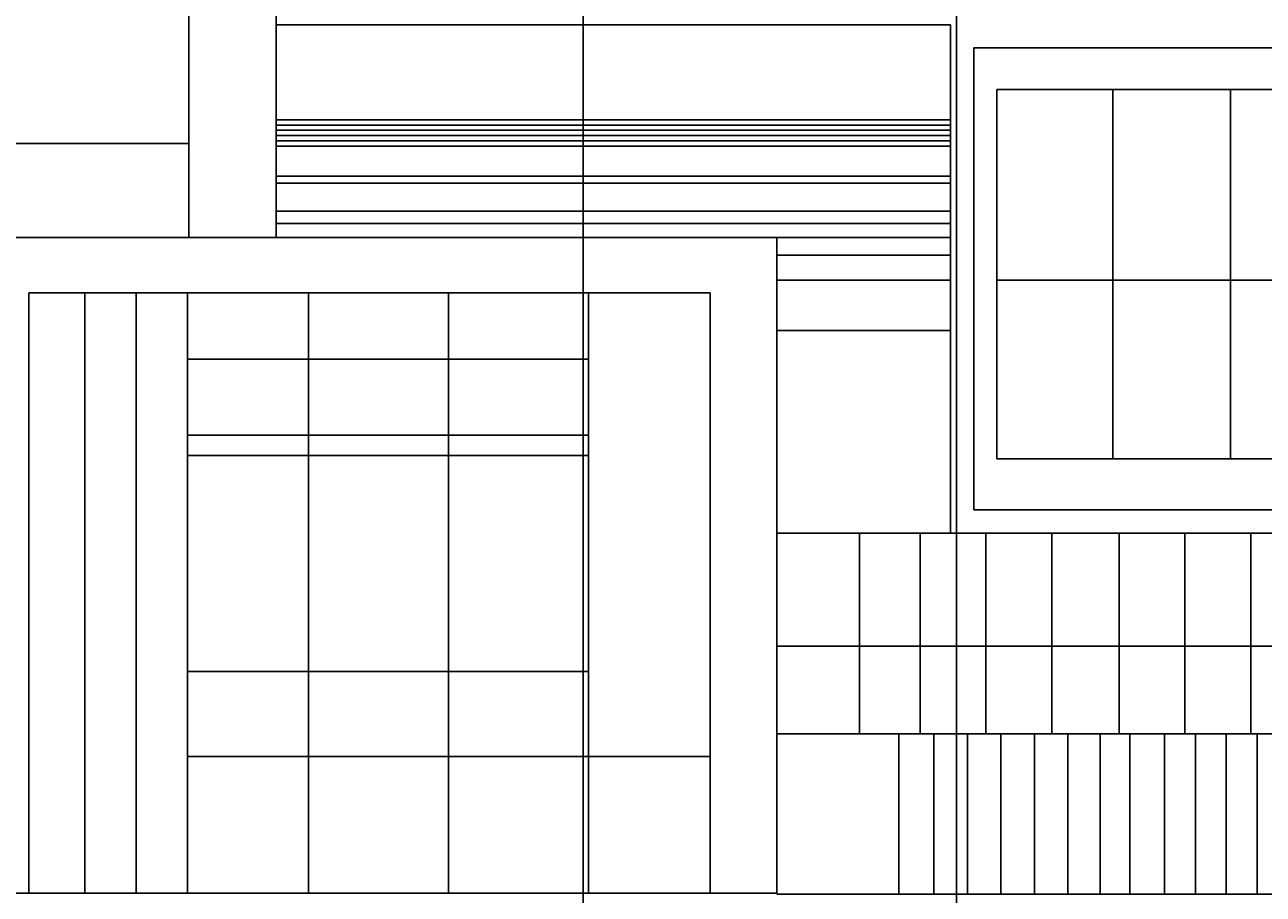
# Model space of a CAD drawing. Units: inches. Extents: x -117 to 121, y -77 to 40.
# Tile 29 of 45: x 9 to 34, y -8 to 10. Entities that reach past the tile are written whole.
import ezdxf

# ---------------------------------------------------------------- set-up
doc = ezdxf.new("R2010")
doc.units = ezdxf.units.IN
doc.header["$MEASUREMENT"] = 0
doc.layers.add('A-ANNO-DIMS', color=2, linetype='Continuous', lineweight=18)
doc.layers.add('A-ELEV', color=7, linetype='Continuous', lineweight=25)
doc.styles.get("Standard").update_dxf_attribs({"font": 'arial.ttf'})
doc.dimstyles.get("Standard").update_dxf_attribs({"dimtxt": 0.18, "dimasz": 0.18, "dimexe": 0.18, "dimexo": 0.0625, "dimgap": 0.09, "dimtad": 0, "dimtih": 1, "dimtoh": 1, "dimdec": 4, "dimzin": 0, "dimdsep": 46, "dimtxsty": 'Standard', "dimcen": 0.09, "dimadec": 0, "dimazin": 0, "dimtfac": 1, "dimtdec": 4, "dimtofl": 0, "dimtmove": 0, "dimatfit": 3, "dimfxl": 1, "dimtolj": 1, "dimtzin": 0, "dimarcsym": 0})

# ---------------------------------------------------------------- blocks, each defined once
blk = doc.blocks.new('*D32')
at = {"layer": 'A-ANNO-DIMS', "color": 0, "lineweight": -2, "transparency": 16777216}
for p, q in [((-3.85, -45.55), (-3.85, 38.61)), ((20.293, -45.55), (20.293, 38.61)), ((-3.67, 38.43), (7.757, 38.43)), ((20.113, 38.43), (8.686, 38.43))]:
    blk.add_line(p, q, dxfattribs=at)
at = {"layer": 'A-ANNO-DIMS', "color": 0, "transparency": 16777216}
for points in [[(-3.67, 38.46), (-3.67, 38.4), (-3.85, 38.43)], [(20.113, 38.46), (20.113, 38.4), (20.293, 38.43)]]:
    blk.add_solid(points, dxfattribs=at)
at = {"layer": 'Defpoints', "color": 0, "transparency": 16777216}
for p in [(20.293, 38.43), (-3.85, -45.613), (20.293, -45.613)]:
    blk.add_point(p, dxfattribs=at)
at = {"layer": 'A-ANNO-DIMS', "color": 0, "transparency": 16777216, "insert": (8.222, 38.43), "char_height": 0.18, "attachment_point": 5}
blk.add_mtext('\\A1;24.142', dxfattribs=at)
blk = doc.blocks.new('*D53')
at = {"layer": 'A-ANNO-DIMS', "color": 0, "lineweight": -2, "transparency": 16777216}
for p, q in [((27.974, 10.841), (27.974, -77.193)), ((51.69, 10.9), (51.69, -77.193)), ((28.154, -77.013), (39.367, -77.013)), ((51.51, -77.013), (40.297, -77.013))]:
    blk.add_line(p, q, dxfattribs=at)
at = {"layer": 'A-ANNO-DIMS', "color": 0, "transparency": 16777216}
for points in [[(28.154, -76.983), (28.154, -77.043), (27.974, -77.013)], [(51.51, -76.983), (51.51, -77.043), (51.69, -77.013)]]:
    blk.add_solid(points, dxfattribs=at)
at = {"layer": 'Defpoints', "color": 0, "transparency": 16777216}
for p in [(51.69, 10.962), (27.974, 10.903), (51.69, -77.013)]:
    blk.add_point(p, dxfattribs=at)
at = {"layer": 'A-ANNO-DIMS', "color": 0, "transparency": 16777216, "insert": (39.832, -77.013), "char_height": 0.18, "attachment_point": 5}
blk.add_mtext('\\A1;23.716', dxfattribs=at)

msp = doc.modelspace()

# ---------------------------------------------------------------- linework, layer by layer
at = {"layer": 'A-ELEV'}
for p, q in [((12.1837, 12.3611), (12.1837, 5.6232)), ((13.9784, 10.755), (13.9784, 5.623)), ((27.8529, 9.9998), (13.9784, 9.9998)), ((27.8529, 9.9998), (27.8529, -0.458)), ((28.3319, 9.5278), (47.4236, 9.5278)), ((28.3319, 9.5278), (28.3319, 0.0223)), ((28.8053, 1.0726), (28.8053, 8.6669)), ((28.8053, 8.6669), (29.2247, 8.6669)), ((29.2247, 8.6669), (35.5042, 8.6669)), ((31.1914, 1.0726), (31.1914, 8.6669)), ((33.6111, 1.0726), (33.6111, 8.6669)), ((27.8529, 8.0465), (13.9784, 8.0465)), ((27.8529, 7.938), (13.9784, 7.938)), ((27.8529, 7.8295), (13.9784, 7.8295)), ((27.8529, 7.721), (13.9784, 7.721)), ((8.5521, 7.5594), (12.1837, 7.5594)), ((27.8529, 7.6124), (13.9784, 7.6124)), ((27.8529, 7.5039), (13.9784, 7.5039)), ((27.8529, 6.889), (13.9784, 6.889)), ((27.8529, 6.7443), (13.9784, 6.7443)), ((27.8529, 6.1656), (13.9784, 6.1656)), ((27.8529, 5.9124), (13.9784, 5.9124)), ((7.6115, 5.6237), (13.9784, 5.623)), ((27.8529, 5.623), (13.9784, 5.623)), ((24.2772, 5.6299), (24.2772, 2.0522)), ((27.8529, 5.2613), (24.2772, 5.2613)), ((24.2772, 4.7497), (27.8529, 4.7497)), ((28.8053, 4.7497), (35.8598, 4.7497)), ((8.8925, -7.8658), (8.8925, 4.4868)), ((8.8925, 4.4868), (22.9063, 4.4868)), ((10.0433, -7.8658), (10.0433, 4.4868)), ((11.0981, -7.8658), (11.0981, 4.4868)), ((12.153, -7.8658), (12.153, 4.4868)), ((14.6462, -7.8658), (14.6462, 4.4868)), ((17.5231, -7.8658), (17.5231, 4.4868)), ((20.3999, -7.8658), (20.3999, 4.4868)), ((22.9063, 4.4868), (22.9063, -7.8658)), ((24.2772, 3.7081), (27.8529, 3.7081)), ((12.153, 3.1214), (20.3999, 3.1214)), ((24.2772, 2.0522), (24.2772, -7.8658)), ((12.153, 1.5596), (20.3999, 1.5596)), ((12.153, 1.1391), (20.3999, 1.1391)), ((35.8598, 1.0726), (28.8053, 1.0726)), ((28.3319, 0.0223), (36.6962, 0.0223)), ((27.8529, -0.458), (24.2772, -0.458)), ((25.9778, -0.458), (25.9778, -4.5859)), ((27.2265, -0.458), (27.2265, -4.5859)), ((27.8529, -0.458), (36.6962, -0.458)), ((28.5793, -0.458), (28.5793, -4.5859)), ((29.9322, -0.458), (29.9322, -4.5859)), ((31.3197, -0.458), (31.3197, -4.5859)), ((32.6725, -0.458), (32.6725, -4.5859)), ((34.0253, -0.458), (34.0253, -4.5859)), ((24.2772, -2.7834), (36.6962, -2.7834)), ((12.153, -3.3062), (20.3999, -3.3062)), ((36.6962, -4.5859), (24.2772, -4.5859)), ((26.7897, -4.5859), (26.7897, -7.8846)), ((27.5071, -4.5859), (27.5071, -7.8846)), ((28.197, -4.5859), (28.197, -7.8846)), ((28.8868, -4.5859), (28.8868, -7.8846)), ((29.5767, -4.5859), (29.5767, -7.8846)), ((30.2666, -4.5859), (30.2666, -7.8846)), ((30.9288, -4.5859), (30.9288, -7.8846)), ((31.5359, -4.5859), (31.5359, -7.8846)), ((32.2533, -4.5859), (32.2533, -7.8846)), ((32.888, -4.5859), (32.888, -7.8846)), ((33.5227, -4.5859), (33.5227, -7.8846)), ((34.1573, -4.5859), (34.1573, -7.8846)), ((12.153, -5.0483), (20.3999, -5.0483)), ((20.3999, -5.0483), (22.9063, -5.0483)), ((7.6115, -7.8658), (8.8925, -7.8658)), ((8.8925, -7.8658), (22.9063, -7.8658)), ((22.9063, -7.8658), (24.2772, -7.8658)), ((41.553, -7.8846), (24.2772, -7.8846))]:
    msp.add_line(p, q, dxfattribs=at)

# ---------------------------------------------------------------- dimensions: what is measured, and where the dimension line sits
at = {"layer": 'A-ANNO-DIMS'}
for base, p1, p2, picture, middle in [((20.2929, 38.4297), (-3.8495, -45.6125), (20.2929, -45.6125), '*D32', (8.2217, 38.4297)), ((51.6901, -77.0135), (27.9744, 10.9032), (51.6901, 10.9623), '*D53', (39.8322, -77.0135))]:
    dim = msp.add_linear_dim(base=base, p1=p1, p2=p2, dimstyle='Standard', override={"dimdec": 3, "dimlfac": 1, "dimrnd": 0, "dimzin": 0, "dimdsep": 46, "dimlunit": 2}, dxfattribs=at)
    dim.commit()
    dim.dimension.update_dxf_attribs({"geometry": picture, "text_midpoint": middle})

doc.saveas('drawing.dxf')
